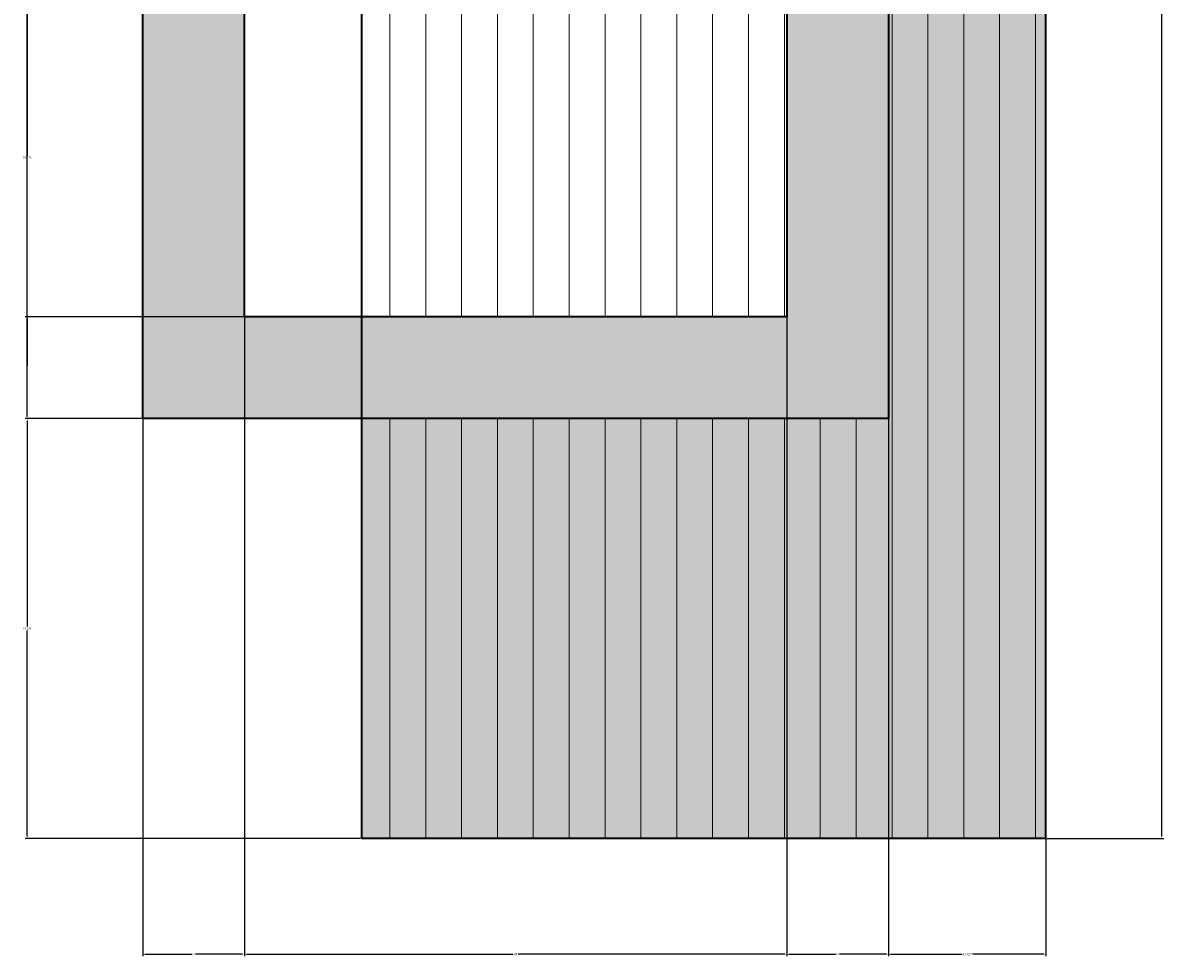
# Model space of a CAD drawing. Units: millimetres. Extents: x 446512 to 447461, y 70395 to 70610.
# Tile 22 of 39: x 446954 to 447055, y 70395 to 70477. Entities that reach past the tile are written whole.
import ezdxf

# ---------------------------------------------------------------- set-up
doc = ezdxf.new("R2010")
doc.units = ezdxf.units.MM
for name, color, linetype, lineweight in [('A-ANNO-DIMS', 2, 'Continuous', 18), ('A-FURN', 7, 'Continuous', 35), ('A-FURN-PATT', 38, 'Continuous', 13)]:
    doc.layers.add(name, color=color, linetype=linetype, lineweight=lineweight)
doc.styles.get("Standard").update_dxf_attribs({"font": 'arial.ttf'})
doc.dimstyles.get("Standard").update_dxf_attribs({"dimtxt": 0.18, "dimasz": 0.18, "dimexe": 0.18, "dimexo": 0.0625, "dimgap": 0.09, "dimtad": 0, "dimtih": 1, "dimtoh": 1, "dimdec": 4, "dimzin": 0, "dimdsep": 46, "dimtxsty": 'Standard', "dimcen": 0.09, "dimadec": 0, "dimazin": 0, "dimtfac": 1, "dimtdec": 4, "dimtofl": 0, "dimtmove": 0, "dimatfit": 3, "dimfxl": 1, "dimtolj": 1, "dimtzin": 0, "dimarcsym": 0})

# ---------------------------------------------------------------- blocks, each defined once
blk = doc.blocks.new('*D46')
at = {"layer": 'A-ANNO-DIMS', "color": 0, "lineweight": -2, "transparency": 16777216}
for p, q in [((446973.17, 70451.39), (446973.17, 70394.88)), ((446964.17, 70442.39), (446964.17, 70394.88)), ((446964.35, 70395.06), (446968.52, 70395.06)), ((446972.99, 70395.06), (446968.82, 70395.06))]:
    blk.add_line(p, q, dxfattribs=at)
at = {"layer": 'A-ANNO-DIMS', "color": 0, "transparency": 16777216}
for points in [[(446964.35, 70395.09), (446964.35, 70395.03), (446964.17, 70395.06)], [(446972.99, 70395.09), (446972.99, 70395.03), (446973.17, 70395.06)]]:
    blk.add_solid(points, dxfattribs=at)
at = {"layer": 'Defpoints', "color": 0, "transparency": 16777216}
for p in [(446973.17, 70451.45), (446964.17, 70442.45), (446973.17, 70395.06)]:
    blk.add_point(p, dxfattribs=at)
at = {"layer": 'A-ANNO-DIMS', "color": 0, "transparency": 16777216, "insert": (446968.67, 70395.06), "char_height": 0.18, "attachment_point": 5}
blk.add_mtext('\\A1;9', dxfattribs=at)
blk = doc.blocks.new('*D47')
at = {"layer": 'A-ANNO-DIMS', "color": 0, "lineweight": -2, "transparency": 16777216}
for p, q in [((446973.17, 70451.39), (446973.17, 70394.88)), ((447021.17, 70451.39), (447021.17, 70394.88)), ((446973.35, 70395.06), (446996.95, 70395.06)), ((447020.99, 70395.06), (446997.39, 70395.06))]:
    blk.add_line(p, q, dxfattribs=at)
at = {"layer": 'A-ANNO-DIMS', "color": 0, "transparency": 16777216}
for points in [[(446973.35, 70395.09), (446973.35, 70395.03), (446973.17, 70395.06)], [(447020.99, 70395.09), (447020.99, 70395.03), (447021.17, 70395.06)]]:
    blk.add_solid(points, dxfattribs=at)
at = {"layer": 'Defpoints', "color": 0, "transparency": 16777216}
for p in [(446973.17, 70451.45), (447021.17, 70451.45), (447021.17, 70395.06)]:
    blk.add_point(p, dxfattribs=at)
at = {"layer": 'A-ANNO-DIMS', "color": 0, "transparency": 16777216, "insert": (446997.17, 70395.06), "char_height": 0.18, "attachment_point": 5}
blk.add_mtext('\\A1;48', dxfattribs=at)
blk = doc.blocks.new('*D48')
at = {"layer": 'A-ANNO-DIMS', "color": 0, "lineweight": -2, "transparency": 16777216}
for p, q in [((447021.17, 70451.39), (447021.17, 70394.88)), ((447030.17, 70442.39), (447030.17, 70394.88)), ((447021.35, 70395.06), (447025.52, 70395.06)), ((447029.99, 70395.06), (447025.82, 70395.06))]:
    blk.add_line(p, q, dxfattribs=at)
at = {"layer": 'A-ANNO-DIMS', "color": 0, "transparency": 16777216}
for points in [[(447021.35, 70395.09), (447021.35, 70395.03), (447021.17, 70395.06)], [(447029.99, 70395.09), (447029.99, 70395.03), (447030.17, 70395.06)]]:
    blk.add_solid(points, dxfattribs=at)
at = {"layer": 'Defpoints', "color": 0, "transparency": 16777216}
for p in [(447021.17, 70451.45), (447030.17, 70442.45), (447030.17, 70395.06)]:
    blk.add_point(p, dxfattribs=at)
at = {"layer": 'A-ANNO-DIMS', "color": 0, "transparency": 16777216, "insert": (447025.67, 70395.06), "char_height": 0.18, "attachment_point": 5}
blk.add_mtext('\\A1;9', dxfattribs=at)
blk = doc.blocks.new('*D49')
at = {"layer": 'A-ANNO-DIMS', "color": 0, "lineweight": -2, "transparency": 16777216}
for p, q in [((447030.17, 70442.39), (447030.17, 70394.88)), ((447044.1, 70405.25), (447044.1, 70394.88)), ((447030.35, 70395.06), (447036.68, 70395.06)), ((447043.92, 70395.06), (447037.59, 70395.06))]:
    blk.add_line(p, q, dxfattribs=at)
at = {"layer": 'A-ANNO-DIMS', "color": 0, "transparency": 16777216}
for points in [[(447030.35, 70395.09), (447030.35, 70395.03), (447030.17, 70395.06)], [(447043.92, 70395.09), (447043.92, 70395.03), (447044.1, 70395.06)]]:
    blk.add_solid(points, dxfattribs=at)
at = {"layer": 'Defpoints', "color": 0, "transparency": 16777216}
for p in [(447030.17, 70442.45), (447044.1, 70405.31), (447044.1, 70395.06)]:
    blk.add_point(p, dxfattribs=at)
at = {"layer": 'A-ANNO-DIMS', "color": 0, "transparency": 16777216, "insert": (447037.13, 70395.06), "char_height": 0.18, "attachment_point": 5}
blk.add_mtext('\\A1;13.927', dxfattribs=at)
blk = doc.blocks.new('*D52')
at = {"layer": 'A-ANNO-DIMS', "color": 0, "lineweight": -2, "transparency": 16777216}
for p, q in [((447044.16, 70599.71), (447054.53, 70599.71)), ((447054.35, 70599.53), (447054.35, 70502.7)), ((447054.35, 70405.49), (447054.35, 70502.33)), ((447044.16, 70405.31), (447054.53, 70405.31))]:
    blk.add_line(p, q, dxfattribs=at)
at = {"layer": 'A-ANNO-DIMS', "color": 0, "transparency": 16777216}
for points in [[(447054.32, 70599.53), (447054.38, 70599.53), (447054.35, 70599.71)], [(447054.32, 70405.49), (447054.38, 70405.49), (447054.35, 70405.31)]]:
    blk.add_solid(points, dxfattribs=at)
at = {"layer": 'Defpoints', "color": 0, "transparency": 16777216}
for p in [(447044.1, 70599.71), (447054.35, 70599.71), (447044.1, 70405.31)]:
    blk.add_point(p, dxfattribs=at)
at = {"layer": 'A-ANNO-DIMS', "color": 0, "transparency": 16777216, "insert": (447054.35, 70502.51), "char_height": 0.18, "attachment_point": 5}
blk.add_mtext('\\A1;194.4', dxfattribs=at)
blk = doc.blocks.new('*D53')
at = {"layer": 'A-ANNO-DIMS', "color": 0, "lineweight": -2, "transparency": 16777216}
for p, q in [((446964.11, 70442.45), (446953.74, 70442.45)), ((446953.92, 70442.27), (446953.92, 70424.06)), ((446953.92, 70405.49), (446953.92, 70423.7)), ((446983.44, 70405.31), (446953.74, 70405.31))]:
    blk.add_line(p, q, dxfattribs=at)
at = {"layer": 'A-ANNO-DIMS', "color": 0, "transparency": 16777216}
for points in [[(446953.89, 70442.27), (446953.95, 70442.27), (446953.92, 70442.45)], [(446953.89, 70405.49), (446953.95, 70405.49), (446953.92, 70405.31)]]:
    blk.add_solid(points, dxfattribs=at)
at = {"layer": 'Defpoints', "color": 0, "transparency": 16777216}
for p in [(446953.92, 70442.45), (446964.17, 70442.45), (446983.51, 70405.31)]:
    blk.add_point(p, dxfattribs=at)
at = {"layer": 'A-ANNO-DIMS', "color": 0, "transparency": 16777216, "insert": (446953.92, 70423.88), "char_height": 0.18, "attachment_point": 5}
blk.add_mtext('\\A1;37.136', dxfattribs=at)
blk = doc.blocks.new('*D54')
at = {"layer": 'A-ANNO-DIMS', "color": 0, "lineweight": -2, "transparency": 16777216}
for p, q in [((446964.11, 70556.45), (446953.74, 70556.45)), ((446953.92, 70556.27), (446953.92, 70499.63)), ((446953.92, 70442.63), (446953.92, 70499.27)), ((446964.11, 70442.45), (446953.74, 70442.45))]:
    blk.add_line(p, q, dxfattribs=at)
at = {"layer": 'A-ANNO-DIMS', "color": 0, "transparency": 16777216}
for points in [[(446953.89, 70556.27), (446953.95, 70556.27), (446953.92, 70556.45)], [(446953.89, 70442.63), (446953.95, 70442.63), (446953.92, 70442.45)]]:
    blk.add_solid(points, dxfattribs=at)
at = {"layer": 'Defpoints', "color": 0, "transparency": 16777216}
for p in [(446953.92, 70556.45), (446964.17, 70556.45), (446964.17, 70442.45)]:
    blk.add_point(p, dxfattribs=at)
at = {"layer": 'A-ANNO-DIMS', "color": 0, "transparency": 16777216, "insert": (446953.92, 70499.45), "char_height": 0.18, "attachment_point": 5}
blk.add_mtext('\\A1;114', dxfattribs=at)
blk = doc.blocks.new('*D56')
at = {"layer": 'A-ANNO-DIMS', "color": 0, "lineweight": -2, "transparency": 16777216}
for p, q in [((446973.11, 70451.45), (446953.74, 70451.45)), ((446953.92, 70451.27), (446953.92, 70447.13)), ((446953.92, 70442.63), (446953.92, 70446.77)), ((446964.11, 70442.45), (446953.74, 70442.45))]:
    blk.add_line(p, q, dxfattribs=at)
at = {"layer": 'A-ANNO-DIMS', "color": 0, "transparency": 16777216}
for points in [[(446953.89, 70451.27), (446953.95, 70451.27), (446953.92, 70451.45)], [(446953.89, 70442.63), (446953.95, 70442.63), (446953.92, 70442.45)]]:
    blk.add_solid(points, dxfattribs=at)
at = {"layer": 'Defpoints', "color": 0, "transparency": 16777216}
for p in [(446953.92, 70451.45), (446973.17, 70451.45), (446964.17, 70442.45)]:
    blk.add_point(p, dxfattribs=at)
at = {"layer": 'A-ANNO-DIMS', "color": 0, "transparency": 16777216, "insert": (446953.92, 70446.95), "char_height": 0.18, "attachment_point": 5}
blk.add_mtext('\\A1;9', dxfattribs=at)
blk = doc.blocks.new('*D57')
at = {"layer": 'A-ANNO-DIMS', "color": 0, "lineweight": -2, "transparency": 16777216}
for p, q in [((446964.11, 70479.63), (446953.74, 70479.63)), ((446953.92, 70479.45), (446953.92, 70465.72)), ((446953.92, 70451.63), (446953.92, 70465.36)), ((446973.11, 70451.45), (446953.74, 70451.45))]:
    blk.add_line(p, q, dxfattribs=at)
at = {"layer": 'A-ANNO-DIMS', "color": 0, "transparency": 16777216}
for points in [[(446953.89, 70479.45), (446953.95, 70479.45), (446953.92, 70479.63)], [(446953.89, 70451.63), (446953.95, 70451.63), (446953.92, 70451.45)]]:
    blk.add_solid(points, dxfattribs=at)
at = {"layer": 'Defpoints', "color": 0, "transparency": 16777216}
for p in [(446953.92, 70479.63), (446964.17, 70479.63), (446973.17, 70451.45)]:
    blk.add_point(p, dxfattribs=at)
at = {"layer": 'A-ANNO-DIMS', "color": 0, "transparency": 16777216, "insert": (446953.92, 70465.54), "char_height": 0.18, "attachment_point": 5}
blk.add_mtext('\\A1;28.176', dxfattribs=at)

msp = doc.modelspace()

# ---------------------------------------------------------------- hatches: boundary and pattern name
at = {"layer": 'A-FURN-PATT'}
h = msp.add_hatch(dxfattribs=at)
h.set_pattern_fill('ANSI31', color=256, angle=45)
h.paths.add_polyline_path([(447044.0961, 70599.7147), (446983.5069, 70599.7147), (446983.5069, 70556.4508), (447030.1693, 70556.4508), (447030.1693, 70442.4508), (446983.5069, 70442.4508), (446983.5069, 70405.3145), (447044.0961, 70405.3145)])
h.paths.add_polyline_path([(447021.1693, 70547.4508), (446983.5069, 70547.4508), (446983.5069, 70451.4508), (447021.1693, 70451.4508)], flags=17)
h = msp.add_hatch(color=256, dxfattribs=at)
h.dxf.hatch_style = 1
h.paths.add_polyline_path([(447021.1693, 70483.6935), (446983.5069, 70483.6935), (446983.5069, 70479.6272), (447021.1693, 70479.6272)], flags=17)
h.paths.add_polyline_path([(447030.1693, 70483.6935), (447021.1693, 70483.6935), (447021.1693, 70479.6272), (447030.1693, 70479.6272)], flags=17)
h.paths.add_polyline_path([(447044.0961, 70599.7147), (446983.5069, 70599.7147), (446983.5069, 70556.4508), (447030.1693, 70556.4508), (447030.1693, 70442.4508), (446983.5069, 70442.4508), (446983.5069, 70405.3145), (447044.0961, 70405.3145)])
h = msp.add_hatch(color=256, dxfattribs=at)
h.dxf.hatch_style = 1
h.paths.add_polyline_path([(446983.5069, 70556.4508), (446964.1693, 70556.4508), (446964.1693, 70442.4508), (446983.5069, 70442.4508), (446983.5069, 70451.4508), (446973.1693, 70451.4508), (446973.1693, 70547.4508), (446983.5069, 70547.4508)])
h.paths.add_polyline_path([(447030.1693, 70556.4508), (446983.5069, 70556.4508), (446983.5069, 70547.4508), (447021.1693, 70547.4508), (447021.1693, 70451.4508), (446983.5069, 70451.4508), (446983.5069, 70442.4508), (447030.1693, 70442.4508)])

# ---------------------------------------------------------------- linework, layer by layer
at = {"layer": 'A-FURN'}
for p, q in [((446983.5069, 70599.7147), (446983.5069, 70405.3145)), ((447044.0961, 70405.3145), (447044.0961, 70599.7147)), ((446983.5069, 70405.3145), (447044.0961, 70405.3145))]:
    msp.add_line(p, q, dxfattribs=at)
for points in [[(447030.1693, 70556.4508), (447030.1693, 70442.4508), (446964.1693, 70442.4508), (446964.1693, 70556.4508)], [(447021.1693, 70547.4508), (447021.1693, 70451.4508), (446973.1693, 70451.4508), (446973.1693, 70547.4508)]]:
    msp.add_lwpolyline(points, close=True, dxfattribs=at)

# ---------------------------------------------------------------- dimensions: what is measured, and where the dimension line sits
at = {"layer": 'A-ANNO-DIMS'}
for base, p1, p2, override, picture, middle in [((447054.3461, 70599.7147), (447044.0961, 70405.3145), (447044.0961, 70599.7147), {"dimdec": 1, "dimlfac": 1, "dimrnd": 0, "dimzin": 0, "dimdsep": 46, "dimlunit": 2}, '*D52', (447054.3461, 70502.5146)), ((446953.9193, 70556.4508), (446964.1693, 70442.4508), (446964.1693, 70556.4508), {"dimdec": 0, "dimlfac": 1, "dimrnd": 0, "dimzin": 0, "dimdsep": 46, "dimlunit": 2}, '*D54', (446953.9193, 70499.4508)), ((446953.9193, 70479.6272), (446973.1693, 70451.4508), (446964.1693, 70479.6272), {"dimdec": 3, "dimlfac": 1, "dimrnd": 0, "dimzin": 0, "dimdsep": 46, "dimlunit": 2}, '*D57', (446953.9193, 70465.539)), ((446953.9193, 70451.4508), (446964.1693, 70442.4508), (446973.1693, 70451.4508), {"dimdec": 0, "dimlfac": 1, "dimrnd": 0, "dimzin": 0, "dimdsep": 46, "dimlunit": 2}, '*D56', (446953.9193, 70446.9508)), ((446953.9193, 70442.4508), (446983.5069, 70405.3145), (446964.1693, 70442.4508), {"dimdec": 3, "dimlfac": 1, "dimrnd": 0, "dimzin": 0, "dimdsep": 46, "dimlunit": 2}, '*D53', (446953.9193, 70423.8826))]:
    dim = msp.add_linear_dim(base=base, p1=p1, p2=p2, angle=90, dimstyle='Standard', override=override, dxfattribs=at)
    dim.commit()
    dim.dimension.update_dxf_attribs({"geometry": picture, "text_midpoint": middle})
for base, p1, p2, override, picture, middle in [((446973.1693, 70395.0645), (446964.1693, 70442.4508), (446973.1693, 70451.4508), {"dimdec": 0, "dimlfac": 1, "dimrnd": 0, "dimzin": 0, "dimdsep": 46, "dimlunit": 2}, '*D46', (446968.6693, 70395.0645)), ((447021.1693, 70395.0645), (446973.1693, 70451.4508), (447021.1693, 70451.4508), {"dimdec": 0, "dimlfac": 1, "dimrnd": 0, "dimzin": 0, "dimdsep": 46, "dimlunit": 2}, '*D47', (446997.1693, 70395.0645)), ((447030.1693, 70395.0645), (447021.1693, 70451.4508), (447030.1693, 70442.4508), {"dimdec": 0, "dimlfac": 1, "dimrnd": 0, "dimzin": 0, "dimdsep": 46, "dimlunit": 2}, '*D48', (447025.6693, 70395.0645)), ((447044.0961, 70395.0645), (447030.1693, 70442.4508), (447044.0961, 70405.3145), {"dimdec": 3, "dimlfac": 1, "dimrnd": 0, "dimzin": 0, "dimdsep": 46, "dimlunit": 2}, '*D49', (447037.1327, 70395.0645))]:
    dim = msp.add_linear_dim(base=base, p1=p1, p2=p2, dimstyle='Standard', override=override, dxfattribs=at)
    dim.commit()
    dim.dimension.update_dxf_attribs({"geometry": picture, "text_midpoint": middle})

doc.saveas('drawing.dxf')
